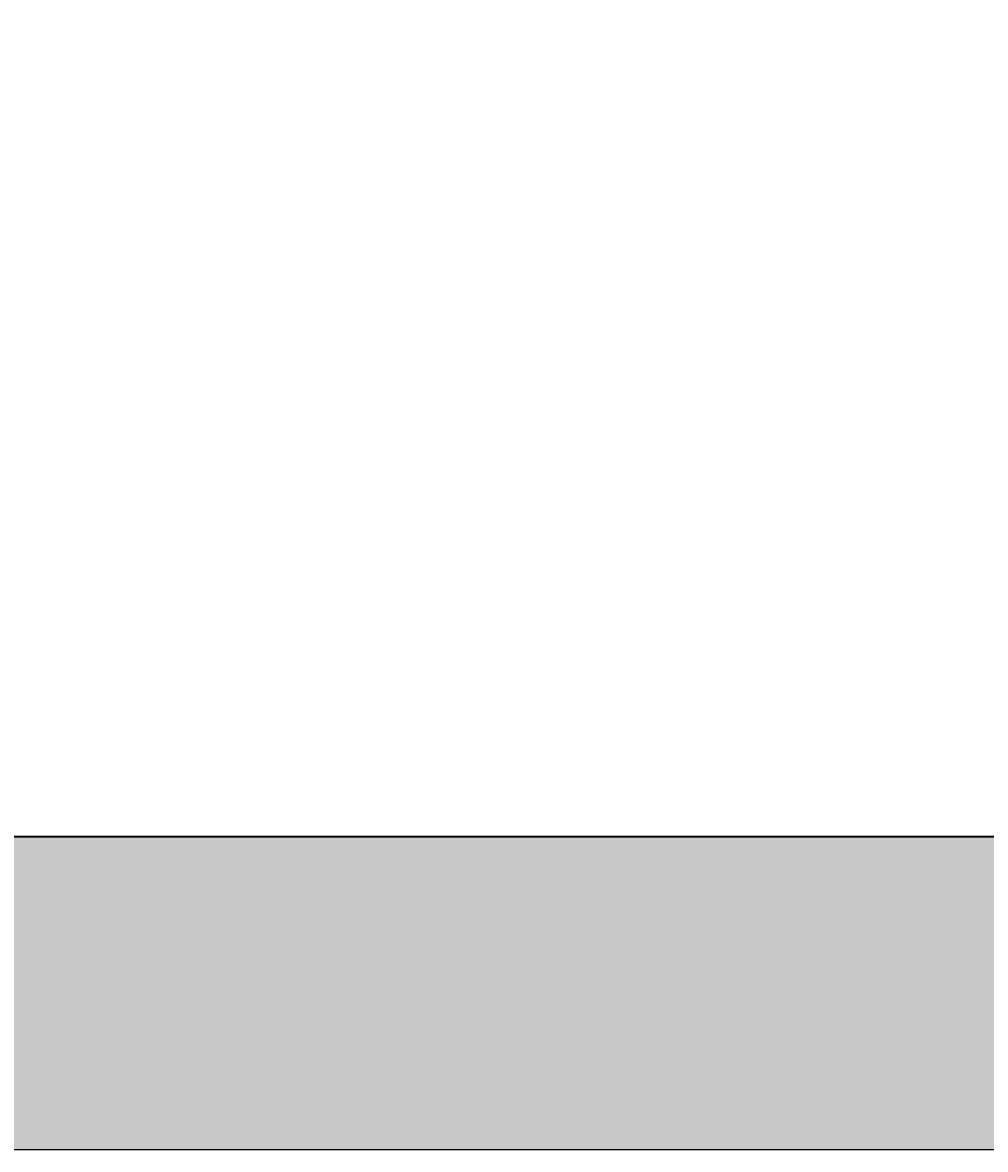
# Model space of a CAD drawing. Units: inches. Extents: x 1998 to 2588, y 1139 to 1977.
# Tile 100 of 134: x 2425 to 2452, y 1523 to 1555. Entities that reach past the tile are written whole.
import ezdxf

# ---------------------------------------------------------------- set-up
doc = ezdxf.new("R2010")
doc.units = ezdxf.units.IN
for name, color, linetype, lineweight in [('A-ANNO-DIMS', 2, 'Continuous', 18), ('A-FLOR-EVTR', 7, 'Continuous', 35), ('A-WALL-PATT', 252, 'Continuous', 13)]:
    doc.layers.add(name, color=color, linetype=linetype, lineweight=lineweight)
doc.styles.get("Standard").update_dxf_attribs({"font": 'arial.ttf'})
doc.dimstyles.get("Standard").update_dxf_attribs({"dimtxt": 0.18, "dimasz": 0.18, "dimexe": 0.18, "dimexo": 0.0625, "dimgap": 0.09, "dimtad": 0, "dimtih": 1, "dimtoh": 1, "dimdec": 4, "dimzin": 0, "dimdsep": 46, "dimtxsty": 'Standard', "dimcen": 0.09, "dimadec": 0, "dimazin": 0, "dimtfac": 1, "dimtdec": 4, "dimtofl": 0, "dimtmove": 0, "dimatfit": 3, "dimfxl": 1, "dimtolj": 1, "dimtzin": 0, "dimarcsym": 0})

# ---------------------------------------------------------------- blocks, each defined once
blk = doc.blocks.new('*D24')
at = {"layer": 'A-ANNO-DIMS', "color": 0, "lineweight": -2, "transparency": 16777216}
for p, q in [((2398.535, 1911.232), (2588.309, 1911.232)), ((2588.129, 1911.052), (2588.129, 1570.164)), ((2588.129, 1228.912), (2588.129, 1569.8)), ((2527.535, 1228.732), (2588.309, 1228.732))]:
    blk.add_line(p, q, dxfattribs=at)
at = {"layer": 'A-ANNO-DIMS', "color": 0, "transparency": 16777216}
for points in [[(2588.099, 1911.052), (2588.159, 1911.052), (2588.129, 1911.232)], [(2588.099, 1228.912), (2588.159, 1228.912), (2588.129, 1228.732)]]:
    blk.add_solid(points, dxfattribs=at)
at = {"layer": 'Defpoints', "color": 0, "transparency": 16777216}
for p in [(2398.473, 1911.232), (2588.129, 1911.232), (2527.473, 1228.732)]:
    blk.add_point(p, dxfattribs=at)
at = {"layer": 'A-ANNO-DIMS', "color": 0, "transparency": 16777216, "insert": (2588.129, 1569.982), "char_height": 0.18, "attachment_point": 5}
blk.add_mtext('\\A1;682.5', dxfattribs=at)
blk = doc.blocks.new('*D42')
at = {"layer": 'A-ANNO-DIMS', "color": 0, "lineweight": -2, "transparency": 16777216}
for p, q in [((2287.535, 1588.732), (2588.309, 1588.732)), ((2588.129, 1588.552), (2588.129, 1555.914)), ((2588.129, 1522.912), (2588.129, 1555.55)), ((2287.535, 1522.732), (2588.309, 1522.732))]:
    blk.add_line(p, q, dxfattribs=at)
at = {"layer": 'A-ANNO-DIMS', "color": 0, "transparency": 16777216}
for points in [[(2588.099, 1588.552), (2588.159, 1588.552), (2588.129, 1588.732)], [(2588.099, 1522.912), (2588.159, 1522.912), (2588.129, 1522.732)]]:
    blk.add_solid(points, dxfattribs=at)
at = {"layer": 'Defpoints', "color": 0, "transparency": 16777216}
for p in [(2287.473, 1588.732), (2588.129, 1588.732), (2287.473, 1522.732)]:
    blk.add_point(p, dxfattribs=at)
at = {"layer": 'A-ANNO-DIMS', "color": 0, "transparency": 16777216, "insert": (2588.129, 1555.732), "char_height": 0.18, "attachment_point": 5}
blk.add_mtext('\\A1;66', dxfattribs=at)

msp = doc.modelspace()

# ---------------------------------------------------------------- hatches: boundary and pattern name
at = {"layer": 'A-WALL-PATT'}
h = msp.add_hatch(color=256, dxfattribs=at)
h.dxf.hatch_style = 1
h.paths.add_polyline_path([(2527.4729, 1362.2324), (2510.9729, 1362.2324), (2510.9729, 1357.7324), (2518.4729, 1357.7324), (2518.4729, 1237.7324), (2503.1458, 1237.7324), (2503.1458, 1228.7324), (2527.4729, 1228.7324)])
h.paths.add_polyline_path([(2490.5682, 1362.2324), (2398.4729, 1362.2324), (2398.4729, 1357.7324), (2490.5682, 1357.7324)])
h.paths.add_polyline_path([(2224.9729, 1264.7324), (2222.9729, 1264.7324), (2222.9729, 1232.4125), (2341.4729, 1232.4125), (2341.4729, 1234.4125), (2224.9729, 1234.4125)])
h.paths.add_polyline_path([(2334.5332, 1273.7324), (2264.7638, 1273.7324), (2264.7638, 1269.5611, -0.043659), (2264.3413, 1264.7324), (2334.5332, 1264.7324)])
h.paths.add_polyline_path([(2236.9551, 1273.7324), (2234.4125, 1273.7324), (2234.4125, 1264.7324), (2236.9551, 1264.7324), (2236.9551, 1269.5611)])
h.paths.add_polyline_path([(2222.9729, 1293.2324), (2096.9729, 1293.2324), (2096.9729, 1345.0966), (2087.9729, 1345.0966), (2087.9729, 1284.2324), (2222.9729, 1284.2324), (2222.9729, 1285.137)])
h.paths.add_polyline_path([(2096.9729, 1458.7927), (2087.9729, 1458.7927), (2087.9729, 1417.7324), (2087.9729, 1413.2324), (2096.9729, 1413.2324), (2096.9729, 1417.7324)])
h.paths.add_polyline_path([(2096.9729, 1413.2324), (2087.9729, 1413.2324), (2087.9729, 1365.5012), (2096.9729, 1365.5012), (2096.9729, 1369.3358)])
h.paths.add_polyline_path([(2186.2943, 1417.7324), (2138.6074, 1417.7324), (2096.9729, 1417.7324), (2096.9729, 1413.2324), (2138.6074, 1413.2324), (2186.2943, 1413.2324)])
h.paths.add_polyline_path([(2181.4729, 1465.7324), (2176.9729, 1465.7324), (2176.9729, 1451.6434), (2181.4729, 1451.6434)])
h.paths.add_polyline_path([(2181.4729, 1422.1664), (2176.9729, 1422.1664), (2176.9729, 1417.7324), (2181.4729, 1417.7324)])
h.paths.add_polyline_path([(2063.9729, 1465.7324), (2087.9729, 1465.7324), (2087.9729, 1470.2324), (2059.4729, 1470.2324), (2059.4729, 1413.2324), (2087.9729, 1413.2324), (2087.9729, 1417.7324), (2063.9729, 1417.7324)])
h.paths.add_polyline_path([(2181.4729, 1755.2324), (2176.9729, 1755.2324), (2176.9729, 1748.6798), (2177.0513, 1748.6798), (2181.4729, 1748.6798)])
h.paths.add_polyline_path([(2227.4729, 1707.2324), (2220.4647, 1707.2324), (2220.4647, 1702.7324), (2222.9729, 1702.7324), (2222.9729, 1604.637), (2227.4729, 1604.637)])
h.paths.add_polyline_path([(2114.9729, 1702.7324), (2105.9729, 1702.7324), (2105.9729, 1628.4781, -0.0318759), (2110.1012, 1628.7416), (2114.9729, 1628.7416)])
h.paths.add_polyline_path([(2345.9729, 1739.3278), (2341.4729, 1739.3278), (2341.4729, 1647.5211), (2345.9729, 1647.5211)])
h.paths.add_polyline_path([(2350.6273, 1641.2324), (2345.9729, 1641.2324), (2345.9729, 1636.7324), (2350.6273, 1636.7324), (2350.6273, 1639.8729)])
h.paths.add_polyline_path([(2501.9729, 1641.2324), (2407.9729, 1641.2324), (2392.5005, 1641.2324), (2392.5005, 1639.8729), (2392.5005, 1636.7324), (2501.9729, 1636.7324)])
h.paths.add_polyline_path([(2510.9729, 1755.2324), (2501.9729, 1755.2324), (2501.9729, 1641.2324), (2510.9729, 1641.2324)])
h.paths.add_polyline_path([(2549.1786, 1641.2324), (2522.3775, 1641.2324), (2522.3775, 1636.7324), (2540.1786, 1636.7324), (2540.1786, 1480.7324), (2522.3775, 1480.7324), (2522.3775, 1476.2324), (2549.1786, 1476.2324)])
h.paths.add_polyline_path([(2498.1786, 1594.7324), (2407.9729, 1594.7324), (2407.9729, 1585.7324), (2416.9729, 1585.7324), (2489.1786, 1585.7324), (2489.1786, 1531.7324), (2416.9729, 1531.7324), (2407.9729, 1531.7324), (2407.9729, 1522.7324), (2498.1786, 1522.7324)])
h.paths.add_polyline_path([(2351.6437, 1480.7324), (2345.9729, 1480.7324), (2345.9729, 1476.2324), (2351.6437, 1476.2324), (2351.6437, 1477.5919)])
h.paths.add_polyline_path([(2501.9729, 1480.7324), (2498.1786, 1480.7324), (2407.9729, 1480.7324), (2393.5168, 1480.7324), (2393.5168, 1477.5919), (2393.5168, 1476.2324), (2501.9729, 1476.2324)])

# ---------------------------------------------------------------- linework, layer by layer
at = {"layer": 'A-FLOR-EVTR'}
msp.add_lwpolyline([(2416.9729, 1531.7324), (2489.1786, 1531.7324), (2489.1786, 1585.7324), (2416.9729, 1585.7324)], dxfattribs=at)

# ---------------------------------------------------------------- dimensions: what is measured, and where the dimension line sits
at = {"layer": 'A-ANNO-DIMS'}
for base, p1, p2, override, picture, middle in [((2588.1286, 1911.2324), (2527.4729, 1228.7324), (2398.4729, 1911.2324), {"dimdec": 1, "dimlfac": 1, "dimrnd": 0, "dimzin": 0, "dimdsep": 46, "dimlunit": 2}, '*D24', (2588.1286, 1569.9824)), ((2588.1286, 1588.7324), (2287.4729, 1522.7324), (2287.4729, 1588.7324), {"dimdec": 0, "dimlfac": 1, "dimrnd": 0, "dimzin": 0, "dimdsep": 46, "dimlunit": 2}, '*D42', (2588.1286, 1555.7324))]:
    dim = msp.add_linear_dim(base=base, p1=p1, p2=p2, angle=90, dimstyle='Standard', override=override, dxfattribs=at)
    dim.commit()
    dim.dimension.update_dxf_attribs({"geometry": picture, "text_midpoint": middle})

doc.saveas('drawing.dxf')
